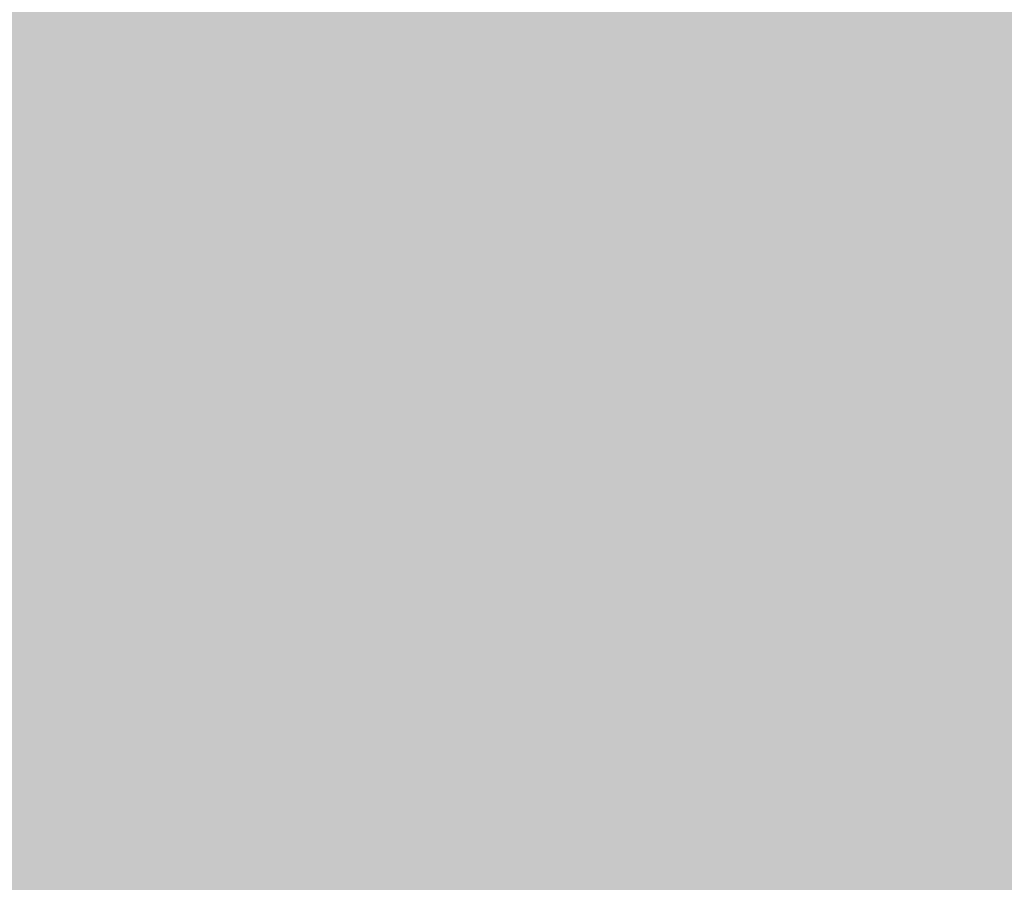
# Model space of a CAD drawing. Units: inches. Extents: x 2083 to 3317, y 1141 to 2115.
# Tile 144 of 256: x 3126.81755 to 3126.89136, y 1263.29018 to 1263.35483. Entities that reach past the tile are written whole.
import ezdxf

# ---------------------------------------------------------------- set-up
doc = ezdxf.new("R2010")
doc.units = ezdxf.units.IN
doc.layers.add('A-ANNO-DIMS', color=2, linetype='Continuous', lineweight=18)
doc.layers.add('A-WALL-PATT', color=251, linetype='Continuous', lineweight=13, true_color=0x636466)
doc.styles.get("Standard").update_dxf_attribs({"font": 'arial.ttf'})
doc.dimstyles.new('ISO-25', dxfattribs={"dimtxt": 12, "dimasz": 12, "dimexe": 1.25, "dimexo": 0.625, "dimtad": 1, "dimlunit": 3, "dimtxsty": 'Standard', "dimcen": 2.5, "dimadec": 0, "dimazin": 0, "dimtfac": 1, "dimtmove": 0, "dimatfit": 3, "dimfxl": 1, "dimarcsym": 0})

# ---------------------------------------------------------------- blocks, each defined once
blk = doc.blocks.new('*D26')
at = {"layer": 'A-ANNO-DIMS', "color": 0, "lineweight": -2, "transparency": 16777216}
for p, q in [((3088.985844, 1274.915092), (3088.985844, 1270.951963)), ((3111.240037, 1274.915092), (3111.240037, 1270.951963)), ((3076.985844, 1272.201963), (2840.262447, 1272.201963)), ((3111.240037, 1272.201963), (3088.985844, 1272.201963)), ((3123.240037, 1272.201963), (3135.240037, 1272.201963))]:
    blk.add_line(p, q, dxfattribs=at)
at = {"layer": 'A-ANNO-DIMS', "color": 0, "transparency": 16777216}
for points in [[(3076.985844, 1274.201963), (3076.985844, 1270.201963), (3088.985844, 1272.201963)], [(3123.240037, 1274.201963), (3123.240037, 1270.201963), (3111.240037, 1272.201963)]]:
    blk.add_solid(points, dxfattribs=at)
at = {"layer": 'Defpoints', "color": 0, "transparency": 16777216}
for p in [(3088.985844, 1275.540092), (3111.240037, 1275.540092), (3088.985844, 1272.201963)]:
    blk.add_point(p, dxfattribs=at)
at = {"layer": 'A-ANNO-DIMS', "color": 0, "transparency": 16777216, "insert": (2952.624146, 1279.031602), "char_height": 12, "attachment_point": 5}
blk.add_mtext('NIGHTSTAND 1\'-10 1/2" TYP.', dxfattribs=at)
blk = doc.blocks.new('*D27')
at = {"layer": 'A-ANNO-DIMS', "color": 0, "lineweight": -2, "transparency": 16777216}
for p, q in [((3114.578165, 1309.794285), (3114.578165, 1321.794285)), ((3111.865037, 1297.794285), (3115.828165, 1297.794285)), ((3114.578165, 1297.794285), (3114.578165, 1275.540092)), ((3111.865037, 1275.540092), (3115.828165, 1275.540092)), ((3114.578165, 1263.540092), (3114.578165, 1140.988591))]:
    blk.add_line(p, q, dxfattribs=at)
at = {"layer": 'A-ANNO-DIMS', "color": 0, "transparency": 16777216}
for points in [[(3112.578165, 1309.794285), (3116.578165, 1309.794285), (3114.578165, 1297.794285)], [(3112.578165, 1263.540092), (3116.578165, 1263.540092), (3114.578165, 1275.540092)]]:
    blk.add_solid(points, dxfattribs=at)
at = {"layer": 'Defpoints', "color": 0, "transparency": 16777216}
for p in [(3111.240037, 1297.794285), (3111.240037, 1275.540092), (3114.578165, 1275.540092)]:
    blk.add_point(p, dxfattribs=at)
at = {"layer": 'A-ANNO-DIMS', "color": 0, "transparency": 16777216, "insert": (3107.748527, 1196.264342), "char_height": 12, "attachment_point": 5, "rotation": 90}
blk.add_mtext('1\'-10 1/2" TYP.', dxfattribs=at)

msp = doc.modelspace()

# ---------------------------------------------------------------- hatches: boundary and pattern name
at = {"layer": 'A-WALL-PATT'}
h = msp.add_hatch(color=256, dxfattribs=at)
h.dxf.hatch_style = 1
h.paths.add_polyline_path([(3126.959783, 2020.76136), (2748.959783, 2020.76136), (2604.959783, 2020.76136), (2226.959783, 2020.76136), (2226.959783, 1702.76136), (2466.959783, 1702.76136), (2466.959783, 1582.76136), (2418.959783, 1582.76136), (2418.959783, 1477.76136), (2226.959783, 1477.76136), (2226.959783, 1263.26136), (2544.959783, 1263.26136), (2544.959783, 1411.76136), (2604.959783, 1411.76136), (2685.959783, 1411.76136), (2685.959783, 1420.76136), (2604.959783, 1420.76136), (2604.959783, 1573.76136), (2604.959783, 1702.76136), (2604.959783, 2011.76136), (2748.959783, 2011.76136), (2748.959783, 1702.76136), (2862.959783, 1702.76136), (2862.959783, 1621.76136), (2871.959783, 1621.76136), (2871.959783, 1702.76136), (2883.959783, 1702.76136), (2883.959783, 1706.939459, -0.026459), (2883.959783, 1711.76136), (2757.959783, 1711.76136), (2757.959783, 1807.76136), (2787.959783, 1807.76136), (2787.959783, 1812.26136), (2757.959783, 1812.26136), (2757.959783, 2011.76136), (2877.959783, 2011.76136), (2877.959783, 1812.26136), (2847.959783, 1812.26136), (2847.959783, 1807.76136), (2889.835742, 1807.76136), (2889.835742, 1812.26136), (2882.459783, 1812.26136), (2882.459783, 2011.76136), (3117.959783, 2011.76136), (3117.959783, 1812.26136), (2937.835742, 1812.26136), (2937.835742, 1807.76136), (2995.709783, 1807.76136), (2995.709783, 1796.117666), (3000.209783, 1796.117666), (3000.209783, 1807.76136), (3117.959783, 1807.76136), (3117.959783, 1711.76136), (3000.209783, 1711.76136), (3000.209783, 1760.117666), (2998.572705, 1760.117666, -0.020711), (2995.709783, 1760.117666), (2995.709783, 1711.76136), (2931.959783, 1711.76136), (2931.959783, 1702.76136), (3126.959783, 1702.76136)])
h.paths.add_polyline_path([(2471.459783, 2011.76136), (2471.459783, 1810.01136), (2462.716936, 1810.01136), (2462.716936, 1805.51136), (2505.959783, 1805.51136), (2505.959783, 1810.01136), (2475.959783, 1810.01136), (2475.959783, 2011.76136), (2595.959783, 2011.76136), (2595.959783, 1810.01136), (2565.959783, 1810.01136), (2565.959783, 1805.51136), (2595.959783, 1805.51136), (2595.959783, 1711.76136), (2235.959783, 1711.76136), (2235.959783, 1805.51136), (2353.709783, 1805.51136), (2353.709783, 1796.054162), (2358.209783, 1796.054162), (2358.209783, 1805.51136), (2414.716936, 1805.51136), (2414.716936, 1810.01136), (2235.959783, 1810.01136), (2235.959783, 2011.76136)], flags=16)
h.paths.add_polyline_path([(2270.204734, 1994.610008), (2270.204734, 1970.610008), (2246.204734, 1970.610008), (2246.204734, 1994.610008)], flags=0)
edge = h.paths.add_edge_path(flags=0)
edge.add_ellipse((2332.027391, 1899.798176), major_axis=(-3.042994, 3.042994), ratio=0.16825245, start_angle=-161.332166, end_angle=-156.307114, ccw=False)
edge.add_ellipse((2333.082037, 1898.74353), major_axis=(-1.054646, 1.054646), ratio=0.4535321, start_angle=-123.371019, end_angle=-94.159107)
edge = h.paths.add_edge_path(flags=0)
edge.add_ellipse((2332.027391, 1968.87629), major_axis=(3.042994, 3.042994), ratio=0.16825245, start_angle=18.667834, end_angle=23.692886)
edge.add_spline(control_points=[(2332.925596, 1970.691105), (2332.226768, 1970.3361), (2330.893709, 1969.658905), (2328.41308, 1970.932138), (2327.203934, 1967.748712), (2324.709596, 1969.955589), (2322.532822, 1967.012354), (2320.012846, 1971.295812), (2317.680308, 1968.157845), (2316.040526, 1967.102047), (2315.426904, 1966.809602)], knot_values=[0, 0, 0, 0, 2.267059, 4.324559, 6.685584, 8.878641, 11.121502, 14.300359, 17.755284, 19.732645, 19.732645, 19.732645, 19.732645], degree=3, periodic=0)
edge.add_ellipse((2332.027391, 1968.87629), major_axis=(3.042994, 3.042994), ratio=0.16825245, start_angle=18.667834, end_angle=23.692886, ccw=False)
edge.add_ellipse((2333.082037, 1969.930936), major_axis=(1.054646, 1.054646), ratio=0.4535321, start_angle=56.628981, end_angle=85.840893, ccw=False)
edge = h.paths.add_edge_path(flags=0)
edge.add_spline(control_points=[(2296.428287, 1967.987908), (2293.627804, 1965.336314), (2287.703624, 1959.727094), (2299.74386, 1949.995699), (2294.532591, 1935.668528), (2290.573228, 1920.603512), (2293.394124, 1909.973691), (2296.185407, 1904.966543)], knot_values=[0.099185, 0.099185, 0.099185, 0.099185, 0.345301, 0.619822, 0.982653, 1.386093, 1.810555, 1.810555, 1.810555, 1.810555], degree=3, periodic=0)
edge.add_spline(control_points=[(2296.185407, 1904.966543), (2297.383582, 1902.6193), (2298.000969, 1901.949312), (2298.55297, 1901.468155)], knot_values=[0.006246, 0.006246, 0.006246, 0.006246, 0.055476, 0.055476, 0.055476, 0.055476], degree=3, periodic=0)
edge.add_spline(control_points=[(2298.55297, 1901.468155), (2297.258612, 1900.923224), (2295.225294, 1900.232126), (2293.060229, 1900.614205), (2292.101423, 1900.788415), (2292.089578, 1900.790568)], knot_values=[0.312835, 0.312835, 0.312835, 0.312835, 0.40178, 0.474987, 0.475903, 0.475903, 0.475903, 0.475903], degree=3, periodic=0)
edge.add_arc((2292.793646, 1904.664109), 3.937008, 215.420897, 259.698179, ccw=False)
edge.add_spline(control_points=[(2289.585314, 1902.382304), (2289.476652, 1902.535087), (2289.36848, 1902.688035), (2289.260865, 1902.84117)], knot_values=[0.102872, 0.102872, 0.102872, 0.102872, 0.116896, 0.116896, 0.116896, 0.116896], degree=3, periodic=0)
edge.add_spline(control_points=[(2289.260865, 1902.84117), (2288.686604, 1902.550192), (2287.640048, 1902.019902), (2285.881337, 1901.873954), (2283.852972, 1901.504352), (2281.719987, 1899.710538), (2278.466991, 1899.492942), (2276.157136, 1901.883202), (2272.258953, 1899.804071), (2267.777605, 1901.843183), (2262.243882, 1900.184033), (2257.414927, 1901.782061), (2254.318374, 1900.72612), (2253.178285, 1900.337343)], knot_values=[0, 0, 0, 0, 1.907977, 3.477176, 5.261074, 7.972851, 11.680248, 13.717921, 16.939592, 22.789562, 27.502503, 33.595215, 37.145618, 37.145618, 37.145618, 37.145618], degree=3, periodic=0)
edge.add_line((2253.178285, 1900.337343), (2250.24424, 1902.84117))
edge.add_line((2250.24424, 1902.84117), (2250.24424, 1965.833296))
edge.add_line((2250.24424, 1965.833296), (2253.178285, 1968.337123))
edge.add_spline(control_points=[(2253.178285, 1968.337123), (2254.318374, 1967.948346), (2257.414927, 1966.892405), (2262.243882, 1968.490433), (2267.777605, 1966.831283), (2271.52673, 1968.537217), (2273.875914, 1967.828289), (2274.206701, 1967.727642)], knot_values=[0, 0, 0, 0, 0.09018, 0.244935, 0.364644, 0.513233, 0.537855, 0.537855, 0.537855, 0.537855], degree=3, periodic=0)
edge.add_arc((2274.352887, 1963.793349), 3.937008, 72.051134, 92.127949, ccw=False)
edge.add_arc((2281.296933, 1985.230003), 18.596298, 252.0511336, 288.5657217)
edge.add_arc((2292.316717, 1956.02888), 12.646081, 71.0267879, 113.7782184, ccw=False)
edge = h.paths.add_edge_path(flags=0)
edge.add_spline(control_points=[(2274.899415, 1951.856195), (2275.066156, 1951.616592), (2275.232687, 1951.376588), (2275.397987, 1951.135855)], knot_values=[1.409916, 1.409916, 1.409916, 1.409916, 1.43159, 1.43159, 1.43159, 1.43159], degree=3, periodic=0)
edge.add_spline(control_points=[(2275.397987, 1951.135855), (2275.792106, 1950.561885), (2276.179231, 1949.983774), (2276.545546, 1949.397103)], knot_values=[1.358238, 1.358238, 1.358238, 1.358238, 1.409916, 1.409916, 1.409916, 1.409916], degree=3, periodic=0)
edge.add_line((2276.545546, 1949.397103), (2277.437289, 1947.862185))
edge.add_spline(control_points=[(2277.437289, 1947.862185), (2276.303834, 1945.673115), (2274.639698, 1942.426882), (2274.631615, 1938.0939), (2272.799124, 1930.85155), (2274.356426, 1943.897046), (2275.947681, 1947.923356), (2276.545546, 1949.397103)], knot_values=[0.005632, 0.005632, 0.005632, 0.005632, 0.186014, 0.266002, 0.357087, 0.59639, 0.739732, 0.739732, 0.739732, 0.739732], degree=3, periodic=0)
edge.add_spline(control_points=[(2276.545546, 1949.397103), (2276.179231, 1949.983774), (2275.792106, 1950.561885), (2275.397987, 1951.135855)], knot_values=[1.358238, 1.358238, 1.358238, 1.358238, 1.409916, 1.409916, 1.409916, 1.409916], degree=3, periodic=0)
edge.add_spline(control_points=[(2275.397987, 1951.135855), (2274.9425, 1950.080452), (2274.20776, 1948.025272), (2273.934602, 1944.851477), (2272.468534, 1937.627489), (2273.466216, 1945.696466), (2274.700615, 1951.059472), (2274.899415, 1951.856195)], knot_values=[0.104364, 0.104364, 0.104364, 0.104364, 0.189636, 0.269624, 0.36071, 0.600013, 0.644622, 0.644622, 0.644622, 0.644622], degree=3, periodic=0)
h.paths.add_polyline_path([(2269.167514, 1963.127573, -0.357527), (2268.170633, 1960.97637, -0.092561), (2268.170633, 1939.436325, -0.357527), (2269.167514, 1937.285122, -0.357527), (2267.01631, 1938.282002, -0.164785), (2254.685581, 1938.282002, -0.357527), (2252.534378, 1937.285122, -0.357527), (2253.531259, 1939.436325, -0.092561), (2253.531259, 1960.97637, -0.357527), (2252.534378, 1963.127573, -0.357527), (2254.685581, 1962.130692, -0.164785), (2267.01631, 1962.130692, -0.357527)], flags=0)
h.paths.add_polyline_path([(2248.874068, 1967.8018), (2248.874068, 1957.02771), (2249.457783, 1957.02771), (2249.457783, 1911.646756), (2248.874068, 1911.646756), (2248.874068, 1900.872666), (2246.511863, 1900.872666, 0.197327), (2244.149658, 1902.456873), (2244.149658, 1966.217592, 0.197327), (2246.511863, 1967.8018)], flags=0)
h.paths.add_polyline_path([(2269.167514, 1931.389344, -0.357527), (2268.170633, 1929.238141, -0.092561), (2268.170633, 1907.698096, -0.357527), (2269.167514, 1905.546893, -0.357527), (2267.01631, 1906.543774, -0.164785), (2254.685581, 1906.543774, -0.357527), (2252.534378, 1905.546893, -0.357527), (2253.531259, 1907.698096, -0.092561), (2253.531259, 1929.238141, -0.357527), (2252.534378, 1931.389344, -0.357527), (2254.685581, 1930.392463, -0.164785), (2267.01631, 1930.392463, -0.357527)], flags=0)
edge = h.paths.add_edge_path(flags=0)
edge.add_spline(control_points=[(2276.196858, 1906.723702), (2276.168144, 1909.028928), (2276.114049, 1913.371852), (2270.598417, 1924.924978), (2273.905175, 1919.012779), (2275.921711, 1916.262063), (2275.47457, 1912.402149), (2277.257874, 1910.380621), (2276.696044, 1908.225036), (2276.646218, 1906.813023), (2276.617825, 1906.008407)], knot_values=[0, 0, 0, 0, 8.61026, 16.221274, 18.843057, 23.804898, 27.440828, 29.356102, 31.203478, 33.650687, 33.650687, 33.650687, 33.650687], degree=3, periodic=0)
edge.add_spline(control_points=[(2276.617825, 1906.008407), (2276.623313, 1905.624144), (2276.497738, 1904.628661), (2275.441779, 1903.854725), (2274.937314, 1903.08045), (2274.85908, 1902.84117)], knot_values=[0.156488, 0.156488, 0.156488, 0.156488, 0.184398, 0.231376, 0.250598, 0.250598, 0.250598, 0.250598], degree=3, periodic=0)
edge.add_line((2274.85908, 1902.84117), (2276.50598, 1902.84117))
edge.add_spline(control_points=[(2276.50598, 1902.84117), (2276.788308, 1903.08494), (2277.665071, 1904.125196), (2278.249538, 1904.340738), (2277.653872, 1908.527387), (2278.15567, 1906.227808), (2278.100464, 1905.285948), (2278.846675, 1904.069005), (2277.856785, 1903.414948), (2277.874191, 1902.99105), (2277.903562, 1902.84117)], knot_values=[0.059574, 0.059574, 0.059574, 0.059574, 0.080753, 0.103741, 0.16972, 0.176036, 0.207137, 0.240474, 0.262341, 0.27366, 0.27366, 0.27366, 0.27366], degree=3, periodic=0)
edge.add_line((2277.903562, 1902.84117), (2280.029825, 1902.84117))
edge.add_spline(control_points=[(2280.029825, 1902.84117), (2279.888221, 1903.088398), (2279.499257, 1903.981551), (2280.152284, 1905.939349), (2278.103615, 1909.657757), (2279.762395, 1907.185285), (2280.3279, 1904.874861), (2280.485109, 1903.48959), (2281.463269, 1903.249432), (2281.758343, 1902.936497), (2281.834036, 1902.84117)], knot_values=[0.013856, 0.013856, 0.013856, 0.013856, 0.034874, 0.088867, 0.107879, 0.126738, 0.158714, 0.193757, 0.217487, 0.226722, 0.226722, 0.226722, 0.226722], degree=3, periodic=0)
edge.add_spline(control_points=[(2281.834036, 1902.84117), (2281.787535, 1902.826703), (2281.647022, 1902.782988), (2281.395527, 1902.85949), (2281.088077, 1902.985242), (2280.720683, 1903.060902), (2280.333451, 1903.025726), (2280.124767, 1902.898879), (2280.029825, 1902.84117)], knot_values=[0, 0, 0, 0, 0.14413, 0.435517, 0.749276, 1.153046, 1.548371, 1.878348, 1.878348, 1.878348, 1.878348], degree=3, periodic=0)
edge.add_line((2280.029825, 1902.84117), (2277.903562, 1902.84117))
edge.add_spline(control_points=[(2277.903562, 1902.84117), (2277.892855, 1902.795855), (2277.865396, 1902.679637), (2277.607479, 1902.687483), (2277.27405, 1902.8007), (2276.837921, 1902.619775), (2276.583807, 1902.789261), (2276.50598, 1902.84117)], knot_values=[0, 0, 0, 0, 0.127189, 0.326199, 0.628009, 1.24357, 1.515331, 1.515331, 1.515331, 1.515331], degree=3, periodic=0)
edge.add_line((2276.50598, 1902.84117), (2274.85908, 1902.84117))
edge.add_spline(control_points=[(2274.85908, 1902.84117), (2274.814437, 1902.898587), (2274.72513, 1903.013446), (2274.493477, 1903.118968), (2274.244285, 1902.960539), (2273.937121, 1903.184942), (2273.614039, 1902.983143), (2273.408316, 1902.883045), (2273.322254, 1902.84117)], knot_values=[0, 0, 0, 0, 0.21843, 0.436957, 0.687977, 0.990379, 1.398396, 1.69185, 1.69185, 1.69185, 1.69185], degree=3, periodic=0)
edge.add_spline(control_points=[(2273.322254, 1902.84117), (2273.61674, 1903.445692), (2274.273998, 1904.538253), (2276.027239, 1904.573702), (2276.206963, 1906.583637), (2276.196858, 1906.723702)], knot_values=[0.012227, 0.012227, 0.012227, 0.012227, 0.059472, 0.106218, 0.134458, 0.134458, 0.134458, 0.134458], degree=3, periodic=0)
h.paths.add_polyline_path([(2270.776054, 1897.789828), (2270.776054, 1873.789828), (2246.776054, 1873.789828), (2246.776054, 1897.789828)], flags=0)
h.paths.add_polyline_path([(2353.709783, 1760.005059), (2353.709783, 1760.054162), (2358.209783, 1760.054162, -0.033729)], flags=0)
h.paths.add_polyline_path([(2321.819119, 1737.529186), (2341.995327, 1737.529186, -0.414214), (2343.203273, 1736.321241), (2343.203273, 1721.020596, -0.414214), (2341.995327, 1719.812651), (2321.819119, 1719.812651, -0.414214), (2320.611173, 1721.020596), (2320.611173, 1736.321241, -0.414214)], flags=0)
h.paths.add_polyline_path([(2324.23501, 1736.321241), (2339.579436, 1736.321241, -0.414214), (2341.995327, 1733.905349), (2341.995327, 1725.44973, -0.414214), (2339.579436, 1723.033839), (2333.680588, 1723.033839), (2333.845317, 1722.045467, -0.870646), (2335.425399, 1721.825893, -0.767327), (2333.922694, 1721.423245), (2331.291024, 1721.423245, -0.767327), (2329.788319, 1721.825893, -0.870646), (2331.368401, 1722.045467), (2331.53313, 1723.033839), (2324.23501, 1723.033839, -0.414214), (2321.819119, 1725.44973), (2321.819119, 1733.905349, -0.414214)], flags=0)
h.paths.add_polyline_path([(2570.483789, 1928.615444), (2589.683789, 1928.615444), (2590.168829, 1928.615444), (2590.168829, 1904.993397), (2570.483789, 1904.993397)], flags=0)
h.paths.add_polyline_path([(2574.447324, 1927.263822, -1), (2572.828836, 1927.263822, -1)], flags=0)
h.paths.add_polyline_path([(2573.089867, 1926.940877), (2573.925032, 1927.776042), (2574.147743, 1927.553332), (2573.312577, 1926.718166)], flags=0)
h.paths.add_polyline_path([(2578.779065, 1919.729618, -1), (2571.591663, 1919.729618, -1)], flags=0)
h.paths.add_polyline_path([(2578.385364, 1919.729618, -1), (2571.985364, 1919.729618, -1)], flags=0)
h.paths.add_polyline_path([(2331.595764, 1729.476216, -1), (2333.617954, 1729.476216, -1)], flags=0)
h.paths.add_polyline_path([(2578.034228, 1927.263822, -1), (2576.41574, 1927.263822, -1)], flags=0)
h.paths.add_polyline_path([(2576.688851, 1927.531089), (2576.911562, 1927.753799), (2577.746728, 1926.918634), (2577.524017, 1926.695923)], flags=0)
h.paths.add_polyline_path([(2578.139065, 1909.859539, -1), (2572.231663, 1909.859539, -1)], flags=0)
h.paths.add_polyline_path([(2577.745364, 1909.859539, -1), (2572.625364, 1909.859539, -1)], flags=0)
h.paths.add_polyline_path([(2583.797718, 1927.263822, -1), (2582.179229, 1927.263822, -1)], flags=0)
h.paths.add_polyline_path([(2582.718649, 1927.753799), (2583.553814, 1926.918634), (2583.331103, 1926.695923), (2582.495938, 1927.531089)], flags=0)
h.paths.add_polyline_path([(2582.495938, 1927.531089), (2582.718649, 1927.753799), (2583.553814, 1926.918634), (2583.331103, 1926.695923)], flags=0)
h.paths.add_polyline_path([(2587.739065, 1920.529618, -1), (2581.831663, 1920.529618, -1)], flags=0)
h.paths.add_polyline_path([(2587.345364, 1920.529618, -1), (2582.225364, 1920.529618, -1)], flags=0)
h.paths.add_polyline_path([(2587.384622, 1927.263822, -1), (2585.766133, 1927.263822, -1)], flags=0)
h.paths.add_polyline_path([(2586.081993, 1926.980247), (2586.917158, 1927.815412), (2587.139869, 1927.592702), (2586.304703, 1926.757536)], flags=0)
h.paths.add_polyline_path([(2588.379065, 1910.659539, -1), (2581.191663, 1910.659539, -1)], flags=0)
h.paths.add_polyline_path([(2587.985364, 1910.659539, -1), (2581.585364, 1910.659539, -1)], flags=0)
h.paths.add_polyline_path([(2417.167729, 1729.477895), (2437.343937, 1729.477895, -0.414214), (2438.551883, 1728.26995), (2438.551883, 1712.969306, -0.414214), (2437.343937, 1711.76136), (2417.167729, 1711.76136, -0.414214), (2415.959783, 1712.969306), (2415.959783, 1728.26995, -0.414214)], flags=0)
h.paths.add_polyline_path([(2419.58362, 1728.26995), (2434.928046, 1728.26995, -0.414214), (2437.343937, 1725.854059), (2437.343937, 1717.39844, -0.414214), (2434.928046, 1714.982548), (2429.029199, 1714.982548), (2429.193927, 1713.994176, -0.870646), (2430.774009, 1713.774603, -0.767327), (2429.271304, 1713.371954), (2426.639634, 1713.371954, -0.767327), (2425.136929, 1713.774603, -0.870646), (2426.717011, 1713.994176), (2426.88174, 1714.982548), (2419.58362, 1714.982548, -0.414214), (2417.167729, 1717.39844), (2417.167729, 1725.854059, -0.414214)], flags=0)
h.paths.add_polyline_path([(2419.58362, 1728.26995), (2434.928046, 1728.26995, -0.414214), (2437.343937, 1725.854059), (2437.343937, 1717.39844, -0.414214), (2434.928046, 1714.982548), (2429.029199, 1714.982548), (2428.358118, 1719.009034), (2427.552821, 1719.009034), (2426.88174, 1714.982548), (2419.58362, 1714.982548, -0.414214), (2417.167729, 1717.39844), (2417.167729, 1725.854059, -0.414214)], flags=0)
h.paths.add_polyline_path([(2426.944374, 1721.424925, -1), (2428.966564, 1721.424925, -1)], flags=0)
h.paths.add_polyline_path([(2475.959783, 1702.76136), (2595.959783, 1702.76136), (2595.959783, 1582.76136), (2475.959783, 1582.76136)], flags=16)
h.paths.add_polyline_path([(2427.959783, 1573.76136), (2595.959783, 1573.76136), (2595.959783, 1468.76136), (2595.959783, 1420.76136), (2384.459783, 1420.76136), (2384.459783, 1468.76136), (2427.959783, 1468.76136)], flags=16)
h.paths.add_polyline_path([(2379.959783, 1468.76136), (2379.959783, 1420.76136), (2235.959783, 1420.76136), (2235.959783, 1468.76136)], flags=16)
h.paths.add_polyline_path([(2317.815996, 1466.695767), (2337.992205, 1466.695767, -0.414214), (2339.20015, 1465.487821), (2339.20015, 1450.187177, -0.414214), (2337.992205, 1448.979232), (2317.815996, 1448.979232, -0.414214), (2316.608051, 1450.187177), (2316.608051, 1465.487821, -0.414214)], flags=0)
h.paths.add_polyline_path([(2320.231887, 1465.487821), (2335.576313, 1465.487821, -0.414214), (2337.992205, 1463.07193), (2337.992205, 1454.616311, -0.414214), (2335.576313, 1452.20042), (2329.677466, 1452.20042), (2329.842195, 1451.212047, -0.870646), (2331.422276, 1450.992474, -0.767327), (2329.919571, 1450.589826), (2327.287902, 1450.589826, -0.767327), (2325.785197, 1450.992474, -0.870646), (2327.365278, 1451.212047), (2327.530007, 1452.20042), (2320.231887, 1452.20042, -0.414214), (2317.815996, 1454.616311), (2317.815996, 1463.07193, -0.414214)], flags=0)
h.paths.add_polyline_path([(2320.231887, 1465.487821), (2335.576313, 1465.487821, -0.414214), (2337.992205, 1463.07193), (2337.992205, 1454.616311, -0.414214), (2335.576313, 1452.20042), (2329.677466, 1452.20042), (2329.006385, 1456.226905), (2328.201088, 1456.226905), (2327.530007, 1452.20042), (2320.231887, 1452.20042, -0.414214), (2317.815996, 1454.616311), (2317.815996, 1463.07193, -0.414214)], flags=0)
h.paths.add_polyline_path([(2327.592641, 1458.642796, -1), (2329.614832, 1458.642796, -1)], flags=0)
h.paths.add_polyline_path([(2244.411744, 1433.340453), (2241.920945, 1433.340453, -0.414214), (2240.017856, 1435.243542), (2240.017856, 1440.952808, -0.414211), (2241.920925, 1442.855897), (2244.411744, 1442.855897, -1.976472)], flags=0)
h.paths.add_polyline_path([(2245.356888, 1434.397536, -0.414214), (2245.356888, 1441.798814, -2.144098)], flags=0)
h.paths.add_polyline_path([(2535.959783, 1416.26136), (2535.959783, 1272.26136), (2235.959783, 1272.26136), (2235.959783, 1416.26136)], flags=16)
h.paths.add_polyline_path([(2260.119561, 1384.292841), (2260.119561, 1362.038649), (2237.865369, 1362.038649), (2237.865369, 1384.292841)], flags=0)
edge = h.paths.add_edge_path(flags=0)
edge.add_line((2318.251847, 1362.093298), (2318.145797, 1362.000973))
edge.add_ellipse((2317.445116, 1360.431044), major_axis=(2.82164, 2.82164), ratio=0.16825245, start_angle=18.667834, end_angle=20.948127, ccw=False)
edge.add_ellipse((2318.423045, 1361.408974), major_axis=(0.977929, 0.977929), ratio=0.4535321, start_angle=56.628981, end_angle=70.226201, ccw=False)
edge = h.paths.add_edge_path(flags=0)
edge.add_line((2319.10737, 1295.571078), (2319.015044, 1295.677128))
edge.add_ellipse((2317.445116, 1296.377809), major_axis=(-2.82164, 2.82164), ratio=0.16825245, start_angle=-161.332166, end_angle=-159.051873, ccw=False)
edge.add_ellipse((2318.423045, 1295.39988), major_axis=(-0.977929, 0.977929), ratio=0.4535321, start_angle=-123.371019, end_angle=-109.773799)
edge = h.paths.add_edge_path(flags=0)
edge.add_spline(control_points=[(2284.210349, 1301.170219), (2284.580688, 1300.444719), (2284.891189, 1299.892024), (2285.159553, 1299.461018)], knot_values=[0.039066, 0.039066, 0.039066, 0.039066, 0.055476, 0.055476, 0.055476, 0.055476], degree=3, periodic=0)
edge.add_line((2285.159553, 1299.461018), (2284.210349, 1301.170219))
edge = h.paths.add_edge_path(flags=0)
edge.add_line((2280.412458, 1297.298013), (2283.369991, 1297.036122))
edge.add_line((2283.369991, 1297.036122), (2286.40569, 1297.92631))
edge.add_spline(control_points=[(2286.40569, 1297.92631), (2285.305487, 1297.463119), (2284.344777, 1297.129151), (2283.369991, 1297.036122)], knot_values=[0.394369, 0.394369, 0.394369, 0.394369, 0.475903, 0.475903, 0.475903, 0.475903], degree=3, periodic=0)
edge.add_spline(control_points=[(2283.369991, 1297.036122), (2283.28139, 1297.027666), (2282.316289, 1296.957336), (2281.312502, 1297.134479), (2280.423441, 1297.296016), (2280.412458, 1297.298013)], knot_values=[0.312835, 0.312835, 0.312835, 0.312835, 0.320246, 0.393453, 0.394369, 0.394369, 0.394369, 0.394369], degree=3, periodic=0)
edge = h.paths.add_edge_path(flags=0)
edge.add_line((2284.435561, 1359.607285), (2280.446291, 1355.328047))
edge.add_line((2280.446291, 1355.328047), (2279.579987, 1351.017754))
edge.add_line((2279.579987, 1351.017754), (2282.412974, 1346.580433))
edge.add_spline(control_points=[(2282.412974, 1346.580433), (2283.153331, 1345.589236), (2284.252896, 1344.028897), (2284.801037, 1342.387167), (2284.935162, 1341.805544)], knot_values=[1.240098, 1.240098, 1.240098, 1.240098, 1.332892, 1.382712, 1.382712, 1.382712, 1.382712], degree=3, periodic=0)
edge.add_spline(control_points=[(2284.935162, 1341.805544), (2285.319108, 1340.1406), (2285.233029, 1338.409204), (2284.909938, 1336.654122)], knot_values=[1.097484, 1.097484, 1.097484, 1.097484, 1.240098, 1.240098, 1.240098, 1.240098], degree=3, periodic=0)
edge.add_spline(control_points=[(2284.909938, 1336.654122), (2284.586848, 1334.89904), (2284.026745, 1333.120272), (2283.462644, 1331.360585)], knot_values=[0.95487, 0.95487, 0.95487, 0.95487, 1.097484, 1.097484, 1.097484, 1.097484], degree=3, periodic=0)
edge.add_line((2283.462644, 1331.360585), (2281.890376, 1326.153357))
edge.add_line((2281.890376, 1326.153357), (2280.756259, 1321.056089))
edge.add_line((2280.756259, 1321.056089), (2280.299205, 1316.001977))
edge.add_line((2280.299205, 1316.001977), (2280.715933, 1310.950068))
edge.add_line((2280.715933, 1310.950068), (2282.028094, 1305.972137))
edge.add_line((2282.028094, 1305.972137), (2284.210349, 1301.170219))
edge.add_spline(control_points=[(2284.210349, 1301.170219), (2283.340731, 1302.730185), (2282.611904, 1304.336493), (2282.028094, 1305.972137)], knot_values=[0.099185, 0.099185, 0.099185, 0.099185, 0.241799, 0.241799, 0.241799, 0.241799], degree=3, periodic=0)
edge.add_spline(control_points=[(2282.028094, 1305.972137), (2281.444283, 1307.60778), (2281.005489, 1309.272759), (2280.715933, 1310.950068)], knot_values=[0.241799, 0.241799, 0.241799, 0.241799, 0.384413, 0.384413, 0.384413, 0.384413], degree=3, periodic=0)
edge.add_spline(control_points=[(2280.715933, 1310.950068), (2280.433241, 1312.587613), (2280.289386, 1314.276959), (2280.298894, 1315.962032), (2280.299205, 1316.001977)], knot_values=[0.384413, 0.384413, 0.384413, 0.384413, 0.523647, 0.527028, 0.527028, 0.527028, 0.527028], degree=3, periodic=0)
edge.add_spline(control_points=[(2280.299205, 1316.001977), (2280.312326, 1317.686955), (2280.477871, 1319.367926), (2280.756259, 1321.056089)], knot_values=[0.527028, 0.527028, 0.527028, 0.527028, 0.669642, 0.669642, 0.669642, 0.669642], degree=3, periodic=0)
edge.add_spline(control_points=[(2280.756259, 1321.056089), (2281.034648, 1322.744252), (2281.42588, 1324.439608), (2281.890376, 1326.153357)], knot_values=[0.669642, 0.669642, 0.669642, 0.669642, 0.812256, 0.812256, 0.812256, 0.812256], degree=3, periodic=0)
edge.add_spline(control_points=[(2281.890376, 1326.153357), (2282.264383, 1327.533251), (2282.78787, 1329.26181), (2283.352751, 1331.01778), (2283.462644, 1331.360585)], knot_values=[0.812256, 0.812256, 0.812256, 0.812256, 0.927087, 0.95487, 0.95487, 0.95487, 0.95487], degree=3, periodic=0)
edge.add_line((2283.462644, 1331.360585), (2284.909938, 1336.654122))
edge.add_line((2284.909938, 1336.654122), (2284.935162, 1341.805544))
edge.add_line((2284.935162, 1341.805544), (2282.412974, 1346.580433))
edge.add_spline(control_points=[(2282.412974, 1346.580433), (2281.275127, 1348.103792), (2280.078447, 1349.570318), (2279.579987, 1351.017754)], knot_values=[1.382712, 1.382712, 1.382712, 1.382712, 1.525326, 1.525326, 1.525326, 1.525326], degree=3, periodic=0)
edge.add_spline(control_points=[(2279.579987, 1351.017754), (2279.443282, 1351.414721), (2279.136312, 1352.856922), (2279.73519, 1354.290385), (2280.446291, 1355.328047)], knot_values=[1.525326, 1.525326, 1.525326, 1.525326, 1.564439, 1.667941, 1.667941, 1.667941, 1.667941], degree=3, periodic=0)
edge.add_spline(control_points=[(2280.446291, 1355.328047), (2281.426113, 1356.757835), (2282.930837, 1358.18256), (2284.435561, 1359.607285)], knot_values=[1.667941, 1.667941, 1.667941, 1.667941, 1.810555, 1.810555, 1.810555, 1.810555], degree=3, periodic=0)
edge.add_arc((2280.623075, 1348.518181), 11.72618, 71.0267879, 113.7782184)
edge.add_arc((2270.404892, 1375.595156), 17.243567, 252.0511336, 288.5657217, ccw=False)
edge.add_arc((2263.965969, 1355.717847), 3.650622, 72.051134, 92.127949)
edge.add_arc((2263.965969, 1355.717847), 3.650622, 92.127949, 177.98513)
edge.add_spline(control_points=[(2260.317604, 1355.846199), (2260.260417, 1354.220668), (2260.551278, 1350.186547), (2262.999344, 1346.766251), (2264.472741, 1344.649024)], knot_values=[1.43159, 1.43159, 1.43159, 1.43159, 1.564144, 1.770695, 1.770695, 1.770695, 1.770695], degree=3, periodic=0)
edge.add_line((2264.472741, 1344.649024), (2264.93559, 1343.98253))
edge.add_spline(control_points=[(2263.801044, 1340.248105), (2263.843238, 1340.514088), (2264.067244, 1341.756465), (2264.512693, 1343.002453), (2264.935047, 1343.981083)], knot_values=[0.53657, 0.53657, 0.53657, 0.53657, 0.559349, 0.644622, 0.644622, 0.644622, 0.644622], degree=3, periodic=0)
edge.add_spline(control_points=[(2264.935047, 1343.981083), (2265.117771, 1343.714975), (2265.298875, 1343.447906), (2265.476756, 1343.179365)], knot_values=[1.384077, 1.384077, 1.384077, 1.384077, 1.409916, 1.409916, 1.409916, 1.409916], degree=3, periodic=0)
edge.add_spline(control_points=[(2265.476756, 1343.179365), (2265.654637, 1342.910823), (2265.829296, 1342.64081), (2265.99913, 1342.368812)], knot_values=[1.358238, 1.358238, 1.358238, 1.358238, 1.384077, 1.384077, 1.384077, 1.384077], degree=3, periodic=0)
edge.add_line((2265.99913, 1342.368812), (2266.826006, 1340.945547))
edge.add_spline(control_points=[(2266.826006, 1340.945547), (2268.894401, 1337.089691), (2271.398173, 1325.843001), (2270.516164, 1310.568557), (2275.919376, 1301.860609), (2277.789511, 1299.19945)], knot_values=[0.116896, 0.116896, 0.116896, 0.116896, 0.472987, 1.050969, 1.313793, 1.313793, 1.313793, 1.313793], degree=3, periodic=0)
edge.add_spline(control_points=[(2277.789511, 1299.19945), (2277.839405, 1299.128452), (2277.889428, 1299.057498), (2277.939572, 1298.986584)], knot_values=[0.109884, 0.109884, 0.109884, 0.109884, 0.116896, 0.116896, 0.116896, 0.116896], degree=3, periodic=0)
edge.add_line((2277.939572, 1298.986584), (2277.788849, 1299.199114))
edge.add_spline(control_points=[(2277.788849, 1299.199114), (2277.256582, 1298.929414), (2276.28635, 1298.437902), (2275.039352, 1298.334419), (2274.38333, 1298.238895), (2274.215254, 1298.209338)], knot_values=[33.12187, 33.12187, 33.12187, 33.12187, 35.029056, 36.598255, 37.144827, 37.144827, 37.144827, 37.144827], degree=3, periodic=0)
edge.add_line((2274.215254, 1298.209338), (2273.073147, 1297.892961))
edge.add_spline(control_points=[(2273.073147, 1297.892961), (2272.322936, 1297.579784), (2271.039151, 1296.510508), (2269.248395, 1296.226062), (2268.4231, 1296.374654)], knot_values=[26.532584, 26.532584, 26.532584, 26.532584, 29.198919, 31.839101, 31.839101, 31.839101, 31.839101], degree=3, periodic=0)
edge.add_line((2268.4231, 1296.374654), (2263.878501, 1297.457534))
edge.add_spline(control_points=[(2263.878501, 1297.457534), (2263.556077, 1297.359435), (2261.860306, 1296.838694), (2260.23878, 1297.282407), (2258.933454, 1297.516461)], knot_values=[15.919551, 15.919551, 15.919551, 15.919551, 16.939592, 21.226067, 21.226067, 21.226067, 21.226067], degree=3, periodic=0)
edge.add_line((2258.933454, 1297.516461), (2254.055233, 1297.32901))
edge.add_spline(control_points=[(2254.055233, 1297.32901), (2253.755525, 1297.295815), (2252.113683, 1297.165174), (2250.461869, 1297.544221), (2249.129686, 1297.667882)], knot_values=[5.306517, 5.306517, 5.306517, 5.306517, 6.276435, 10.613034, 10.613034, 10.613034, 10.613034], degree=3, periodic=0)
edge.add_line((2249.129686, 1297.667882), (2244.33165, 1296.877756))
edge.add_line((2244.33165, 1296.877756), (2241.611033, 1299.19945))
edge.add_line((2241.611033, 1299.19945), (2241.611033, 1357.609404))
edge.add_line((2241.611033, 1357.609404), (2244.33165, 1359.931097))
edge.add_line((2244.33165, 1359.931097), (2252.728823, 1359.542692))
edge.add_spline(control_points=[(2252.728823, 1359.542692), (2252.870939, 1359.54644), (2253.30574, 1359.548172), (2253.739845, 1359.514274), (2254.031742, 1359.482426)], knot_values=[0.233291, 0.233291, 0.233291, 0.233291, 0.244935, 0.268927, 0.268927, 0.268927, 0.268927], degree=3, periodic=0)
edge.add_line((2254.031742, 1359.482426), (2259.58719, 1359.41639))
edge.add_spline(control_points=[(2259.58719, 1359.41639), (2260.677068, 1359.628503), (2262.073197, 1359.897003), (2263.523692, 1359.459278), (2263.830417, 1359.365952)], knot_values=[0.422516, 0.422516, 0.422516, 0.422516, 0.513233, 0.537855, 0.537855, 0.537855, 0.537855], degree=3, periodic=0)
edge.add_arc((2263.965969, 1355.717847), 3.650622, 72.051134, 92.127949, ccw=False)
edge.add_arc((2270.404892, 1375.595156), 17.243567, 252.0511336, 288.5657217)
edge.add_arc((2280.623075, 1348.518181), 11.72618, 71.0267879, 113.7782184, ccw=False)
h.paths.add_polyline_path([(2240.34053, 1359.434715), (2240.34053, 1349.444353), (2240.881785, 1349.444353), (2240.881785, 1307.3645), (2240.34053, 1307.3645), (2240.34053, 1297.374138), (2238.150157, 1297.374138, 0.197327), (2235.959783, 1298.843108), (2235.959783, 1357.965746, 0.197327), (2238.150157, 1359.434715)], flags=0)
h.paths.add_polyline_path([(2259.15779, 1355.1005, -0.357527), (2258.233425, 1353.10578, -0.092561), (2258.233425, 1333.132601, -0.357527), (2259.15779, 1331.13788, -0.357527), (2257.16307, 1332.062246, -0.164785), (2245.729302, 1332.062246, -0.357527), (2243.734582, 1331.13788, -0.357527), (2244.658947, 1333.132601, -0.092561), (2244.658947, 1353.10578, -0.357527), (2243.734582, 1355.1005, -0.357527), (2245.729302, 1354.176135, -0.164785), (2257.16307, 1354.176135, -0.357527)], flags=0)
edge = h.paths.add_edge_path(flags=0)
edge.add_line((2265.99913, 1342.368812), (2266.826006, 1340.945547))
edge.add_line((2266.826006, 1340.945547), (2265.307557, 1337.814066))
edge.add_line((2265.307557, 1337.814066), (2264.358232, 1334.652939))
edge.add_line((2264.358232, 1334.652939), (2264.262012, 1333.799705))
edge.add_spline(control_points=[(2264.262012, 1333.799705), (2264.208357, 1333.187055), (2264.16206, 1332.365525), (2264.007144, 1331.413933), (2263.969049, 1331.201834)], knot_values=[0.464444, 0.464444, 0.464444, 0.464444, 0.516691, 0.531608, 0.531608, 0.531608, 0.531608], degree=3, periodic=0)
edge.add_spline(control_points=[(2263.969049, 1331.201834), (2263.774535, 1330.118873), (2263.42437, 1328.790839), (2263.25742, 1328.530652), (2263.234028, 1328.514612)], knot_values=[0.372682, 0.372682, 0.372682, 0.372682, 0.44885, 0.464444, 0.464444, 0.464444, 0.464444], degree=3, periodic=0)
edge.add_spline(control_points=[(2263.234028, 1328.514612), (2263.096382, 1328.420227), (2263.13117, 1329.301477), (2263.274953, 1330.615749)], knot_values=[0.280919, 0.280919, 0.280919, 0.280919, 0.372682, 0.372682, 0.372682, 0.372682], degree=3, periodic=0)
edge.add_spline(control_points=[(2263.274953, 1330.615749), (2263.418736, 1331.930022), (2263.671515, 1333.677318), (2263.969852, 1335.315027)], knot_values=[0.189157, 0.189157, 0.189157, 0.189157, 0.280919, 0.280919, 0.280919, 0.280919], degree=3, periodic=0)
edge.add_spline(control_points=[(2263.969852, 1335.315027), (2264.100496, 1336.032192), (2264.418783, 1337.621911), (2264.754848, 1338.86443), (2264.947419, 1339.491124)], knot_values=[0.097394, 0.097394, 0.097394, 0.097394, 0.137578, 0.189157, 0.189157, 0.189157, 0.189157], degree=3, periodic=0)
edge.add_spline(control_points=[(2264.947419, 1339.491124), (2265.290017, 1340.606055), (2265.644238, 1341.493996), (2265.99913, 1342.368812)], knot_values=[0.005632, 0.005632, 0.005632, 0.005632, 0.097394, 0.097394, 0.097394, 0.097394], degree=3, periodic=0)
h.paths.add_polyline_path([(2259.15779, 1325.670973, -0.357527), (2258.233425, 1323.676253, -0.092561), (2258.233425, 1303.703073, -0.357527), (2259.15779, 1301.708353, -0.357527), (2257.16307, 1302.632719, -0.164785), (2245.729302, 1302.632719, -0.357527), (2243.734582, 1301.708353, -0.357527), (2244.658947, 1303.703073, -0.092561), (2244.658947, 1323.676253, -0.357527), (2243.734582, 1325.670973, -0.357527), (2245.729302, 1324.746608, -0.164785), (2257.16307, 1324.746608, -0.357527)], flags=0)
edge = h.paths.add_edge_path(flags=0)
edge.add_spline(control_points=[(2261.708938, 1317.311421), (2261.679482, 1317.41758), (2261.761858, 1317.388535), (2262.490736, 1316.089873), (2262.962185, 1315.300897)], knot_values=[14.955861, 14.955861, 14.955861, 14.955861, 16.221274, 18.694826, 18.694826, 18.694826, 18.694826], degree=3, periodic=0)
edge.add_spline(control_points=[(2262.962185, 1315.300897), (2262.990437, 1315.253617), (2263.702096, 1314.067376), (2264.348983, 1313.127153), (2264.730054, 1312.164154)], knot_values=[18.694826, 18.694826, 18.694826, 18.694826, 18.843057, 22.433791, 22.433791, 22.433791, 22.433791], degree=3, periodic=0)
edge.add_spline(control_points=[(2264.730054, 1312.164154), (2264.875565, 1311.796437), (2265.176873, 1310.769807), (2265.143069, 1309.559262), (2265.247736, 1308.824193)], knot_values=[22.433791, 22.433791, 22.433791, 22.433791, 23.804898, 26.172756, 26.172756, 26.172756, 26.172756], degree=3, periodic=0)
edge.add_line((2265.247736, 1308.824193), (2265.850774, 1307.171888))
edge.add_spline(control_points=[(2265.850774, 1307.171888), (2266.065025, 1306.821678), (2266.384387, 1306.332246), (2266.4244, 1305.780549), (2266.420369, 1305.611216)], knot_values=[28.062562, 28.062562, 28.062562, 28.062562, 29.356102, 29.911721, 29.911721, 29.911721, 29.911721], degree=3, periodic=0)
edge.add_spline(control_points=[(2266.420369, 1305.611216), (2266.416116, 1305.43259), (2266.393999, 1305.249998), (2266.364777, 1305.065857)], knot_values=[29.911721, 29.911721, 29.911721, 29.911721, 30.497837, 30.497837, 30.497837, 30.497837], degree=3, periodic=0)
edge.add_line((2266.364777, 1305.065857), (2266.066151, 1302.136295))
edge.add_spline(control_points=[(2266.066151, 1302.136295), (2266.07124, 1301.779984), (2265.998076, 1301.199985), (2265.663266, 1300.758961), (2265.508908, 1300.585882)], knot_values=[0.156488, 0.156488, 0.156488, 0.156488, 0.184398, 0.203543, 0.203543, 0.203543, 0.203543], degree=3, periodic=0)
edge.add_line((2265.508908, 1300.585882), (2264.435341, 1299.19945))
edge.add_line((2264.435341, 1299.19945), (2265.962442, 1299.19945))
edge.add_line((2265.962442, 1299.19945), (2267.33599, 1301.175276))
edge.add_line((2267.33599, 1301.175276), (2267.311667, 1301.986237))
edge.add_spline(control_points=[(2267.311667, 1301.986237), (2267.261111, 1302.862396), (2267.160212, 1303.737132), (2267.271486, 1303.325896)], knot_values=[0.126229, 0.126229, 0.126229, 0.126229, 0.166617, 0.166617, 0.166617, 0.166617], degree=3, periodic=0)
edge.add_spline(control_points=[(2267.271486, 1303.325896), (2267.280035, 1303.294305), (2267.309785, 1303.175366), (2267.37345, 1302.883608), (2267.406123, 1302.682829), (2267.417926, 1302.601025)], knot_values=[0.166617, 0.166617, 0.166617, 0.166617, 0.16972, 0.176036, 0.180765, 0.180765, 0.180765, 0.180765], degree=3, periodic=0)
edge.add_spline(control_points=[(2267.743891, 1300.987505), (2267.687583, 1301.150943), (2267.48052, 1301.656664), (2267.483751, 1302.144788), (2267.417926, 1302.601025)], knot_values=[0.180765, 0.180765, 0.180765, 0.180765, 0.193767, 0.220139, 0.220139, 0.220139, 0.220139], degree=3, periodic=0)
edge.add_line((2267.417926, 1302.601025), (2267.743891, 1300.987505))
edge.add_spline(control_points=[(2267.743891, 1300.987505), (2267.831961, 1300.731878), (2267.932021, 1300.309904), (2267.554841, 1299.974518), (2267.429366, 1299.829207)], knot_values=[0.220139, 0.220139, 0.220139, 0.220139, 0.240474, 0.25489, 0.25489, 0.25489, 0.25489], degree=3, periodic=0)
edge.add_line((2267.429366, 1299.829207), (2267.258361, 1299.19945))
edge.add_line((2267.258361, 1299.19945), (2269.229956, 1299.19945))
edge.add_spline(control_points=[(2269.229956, 1299.19945), (2269.098653, 1299.428694), (2268.842774, 1300.016251), (2269.011575, 1300.915923), (2268.946796, 1301.66074)], knot_values=[0.013856, 0.013856, 0.013856, 0.013856, 0.034874, 0.067073, 0.067073, 0.067073, 0.067073], degree=3, periodic=0)
edge.add_line((2268.946796, 1301.66074), (2268.431582, 1303.603109))
edge.add_spline(control_points=[(2268.431582, 1303.603109), (2268.175596, 1304.192375), (2267.596214, 1305.251298), (2268.040698, 1304.62321), (2268.251394, 1304.282421)], knot_values=[0.090155, 0.090155, 0.090155, 0.090155, 0.107879, 0.120289, 0.120289, 0.120289, 0.120289], degree=3, periodic=0)
edge.add_spline(control_points=[(2268.251394, 1304.282421), (2268.360882, 1304.105329), (2269.057753, 1302.917983), (2269.382691, 1301.590419), (2269.521405, 1300.775931), (2269.57522, 1300.555784)], knot_values=[0.120289, 0.120289, 0.120289, 0.120289, 0.126738, 0.158714, 0.173506, 0.173506, 0.173506, 0.173506], degree=3, periodic=0)
edge.add_line((2269.57522, 1300.555784), (2270.685798, 1299.421258))
edge.add_spline(control_points=[(2270.685798, 1299.421258), (2270.767221, 1299.357251), (2270.837852, 1299.281401), (2270.902925, 1299.19945)], knot_values=[0.21816, 0.21816, 0.21816, 0.21816, 0.226722, 0.226722, 0.226722, 0.226722], degree=3, periodic=0)
edge.add_line((2270.937201, 1299.192913), (2270.902925, 1299.19945))
edge.add_spline(control_points=[(2270.902925, 1299.19945), (2270.859806, 1299.186035), (2270.729515, 1299.1455), (2270.496314, 1299.216437), (2270.271661, 1299.308323), (2270.121017, 1299.347961), (2270.063339, 1299.359557)], knot_values=[0.939174, 0.939174, 0.939174, 0.939174, 1.083304, 1.374691, 1.68845, 1.878348, 1.878348, 1.878348, 1.878348], degree=3, periodic=0)
edge.add_line((2270.063339, 1299.359557), (2269.229956, 1299.19945))
edge.add_line((2269.229956, 1299.19945), (2267.258361, 1299.19945))
edge.add_spline(control_points=[(2267.258361, 1299.19945), (2267.248433, 1299.157431), (2267.222971, 1299.049667), (2266.983816, 1299.056942), (2266.80921, 1299.11623), (2266.676905, 1299.109091), (2266.636531, 1299.104815)], knot_values=[0.757665, 0.757665, 0.757665, 0.757665, 0.884854, 1.083864, 1.385675, 1.515331, 1.515331, 1.515331, 1.515331], degree=3, periodic=0)
edge.add_spline(control_points=[(2266.636531, 1299.104815), (2266.485225, 1299.088788), (2266.235807, 1299.017123), (2266.034608, 1299.151317), (2265.962442, 1299.19945)], knot_values=[0, 0, 0, 0, 0.485905, 0.757665, 0.757665, 0.757665, 0.757665], degree=3, periodic=0)
edge.add_line((2265.962442, 1299.19945), (2264.435341, 1299.19945))
edge.add_line((2264.435341, 1299.19945), (2263.858444, 1299.367118))
edge.add_spline(control_points=[(2263.858444, 1299.367118), (2263.818943, 1299.370905), (2263.779528, 1299.385721), (2263.740131, 1299.401504)], knot_values=[0.845925, 0.845925, 0.845925, 0.845925, 0.978627, 0.978627, 0.978627, 0.978627], degree=3, periodic=0)
edge.add_line((2263.721786, 1299.396425), (2263.010306, 1299.19945))
edge.add_spline(control_points=[(2263.010306, 1299.19945), (2263.245794, 1299.682859), (2263.506032, 1300.128107), (2263.873494, 1300.408028)], knot_values=[0.012227, 0.012227, 0.012227, 0.012227, 0.052971, 0.052971, 0.052971, 0.052971], degree=3, periodic=0)
edge.add_spline(control_points=[(2263.873494, 1300.408028), (2263.932131, 1300.452695), (2264.084243, 1300.552979), (2264.255189, 1300.624223), (2264.359686, 1300.664747)], knot_values=[0.052971, 0.052971, 0.052971, 0.052971, 0.059472, 0.069086, 0.069086, 0.069086, 0.069086], degree=3, periodic=0)
edge.add_line((2264.359686, 1300.664747), (2265.1419, 1301.077774))
edge.add_line((2265.1419, 1301.077774), (2265.675806, 1302.799558))
edge.add_line((2265.675806, 1302.799558), (2265.5407, 1305.704066))
edge.add_line((2265.5407, 1305.704066), (2264.803073, 1309.327724))
edge.add_line((2264.803073, 1309.327724), (2263.040535, 1314.091791))
edge.add_spline(control_points=[(2263.040535, 1314.091791), (2262.383572, 1315.671438), (2261.795972, 1316.997749), (2261.708938, 1317.311421)], knot_values=[11.216896, 11.216896, 11.216896, 11.216896, 14.955861, 14.955861, 14.955861, 14.955861], degree=3, periodic=0)
h.paths.add_polyline_path([(2871.959783, 1416.26136), (2895.910047, 1416.26136), (2895.910047, 1420.76136), (2871.959783, 1420.76136), (2871.959783, 1501.76136), (2862.959783, 1501.76136), (2862.959783, 1420.76136), (2805.959783, 1420.76136), (2805.959783, 1411.76136), (2862.959783, 1411.76136), (2862.959783, 1263.26136), (3126.959783, 1263.26136), (3126.959783, 1411.76136), (3126.959783, 1486.76136), (2943.959783, 1486.76136), (2943.959783, 1477.76136), (2967.860311, 1477.76136), (2967.860311, 1420.76136), (2943.910047, 1420.76136), (2943.910047, 1416.26136), (3117.959783, 1416.26136), (3117.959783, 1420.76136), (2972.360311, 1420.76136), (2972.360311, 1477.76136), (3117.959783, 1477.76136), (3117.959783, 1420.76136), (3117.959783, 1272.26136), (2871.959783, 1272.26136)], flags=0)
h.paths.add_polyline_path([(2457.125626, 1485.942505), (2527.602651, 1485.942505), (2527.602651, 1537.635702), (2457.125626, 1537.635702)], flags=8)
h.paths.add_polyline_path([(2481.005058, 1609.981804), (2590.765818, 1609.981804), (2590.765818, 1682.003362), (2481.005058, 1682.003362)], flags=8)
h.paths.add_polyline_path([(2483.085022, 1729.126784), (2553.562048, 1729.126784), (2553.562048, 1780.81998), (2483.085022, 1780.81998)], flags=8)
h = msp.add_hatch(color=256, dxfattribs=at)
h.dxf.hatch_style = 1
h.paths.add_polyline_path([(3126.959783, 1486.76136), (2943.959783, 1486.76136), (2943.959783, 1477.76136), (2967.860311, 1477.76136), (2967.860311, 1420.76136), (2943.910047, 1420.76136), (2943.910047, 1416.26136), (3117.959783, 1416.26136), (3117.959783, 1420.76136), (2972.360311, 1420.76136), (2972.360311, 1477.76136), (3117.959783, 1477.76136), (3117.959783, 1420.76136), (3117.959783, 1272.26136), (2871.959783, 1272.26136), (2871.959783, 1416.26136), (2895.910047, 1416.26136), (2895.910047, 1420.76136), (2871.959783, 1420.76136), (2871.959783, 1501.76136), (2862.959783, 1501.76136), (2862.959783, 1420.76136), (2805.959783, 1420.76136), (2805.959783, 1411.76136), (2862.959783, 1411.76136), (2862.959783, 1263.26136), (3126.959783, 1263.26136), (3126.959783, 1411.76136)])

# ---------------------------------------------------------------- dimensions: what is measured, and where the dimension line sits
at = {"layer": 'A-ANNO-DIMS'}
for base, p1, p2, angle, text, picture, middle in [((3114.578165, 1275.540092), (3111.240037, 1297.794285), (3111.240037, 1275.540092), 270, '<> TYP.', '*D27', (3107.748527, 1196.264342)), ((3088.985844, 1272.201963), (3111.240037, 1275.540092), (3088.985844, 1275.540092), 180, 'NIGHTSTAND <> TYP.', '*D26', (2952.624146, 1279.031602))]:
    dim = msp.add_linear_dim(base=base, p1=p1, p2=p2, angle=angle, text=text, dimstyle='ISO-25', override={"dimdec": 1, "dimlfac": 1, "dimrnd": 0, "dimzin": 1, "dimdsep": 46, "dimlunit": 4, "dimfrac": 2}, dxfattribs=at)
    dim.commit()
    dim.dimension.update_dxf_attribs({"geometry": picture, "text_midpoint": middle})

doc.saveas('drawing.dxf')
